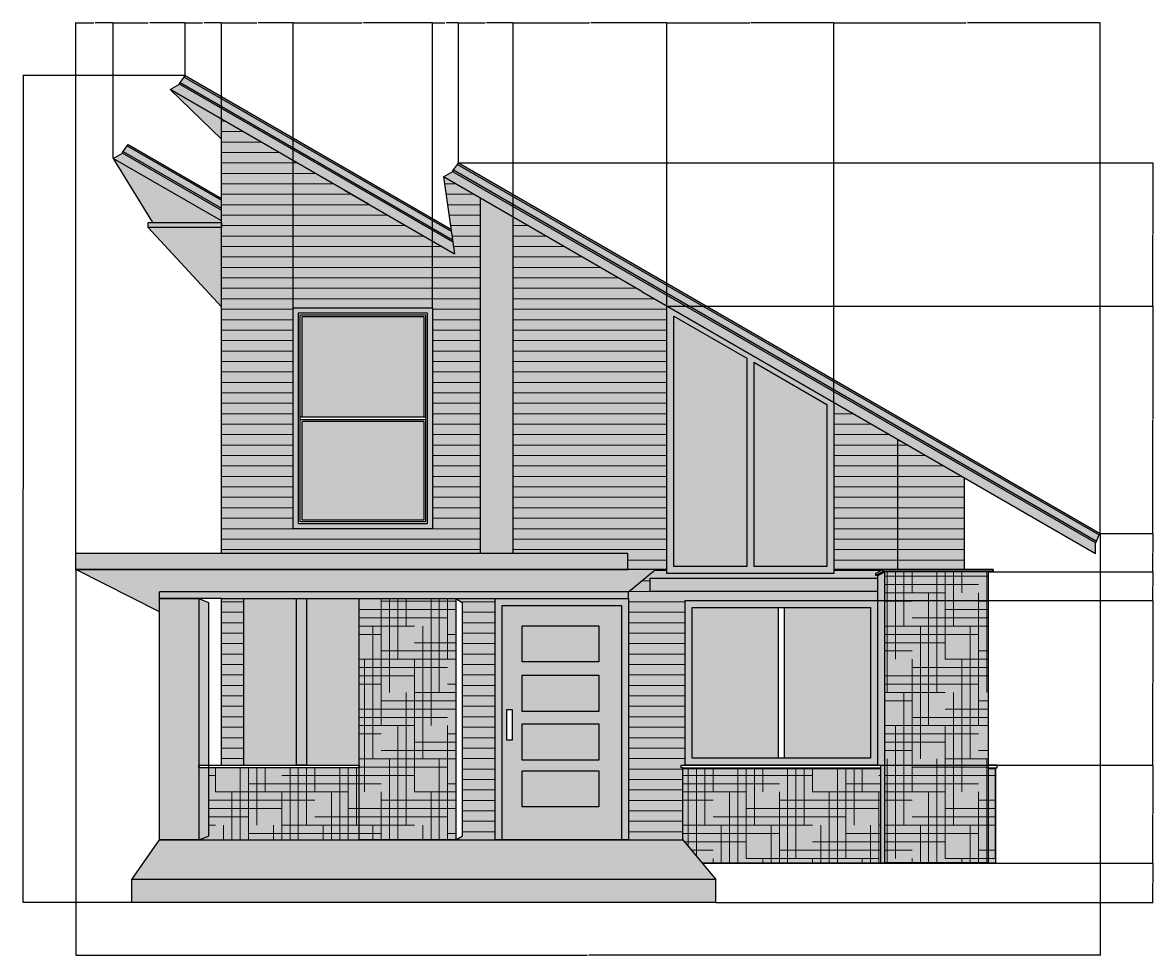
# Model space of a CAD drawing. Units: millimetres. Extents: x 171 to 1599, y 973 to 1509.
# Tile 1 of 7: x 171 to 821, y 973 to 1509. Entities that reach past the tile are written whole.
import ezdxf

# ---------------------------------------------------------------- set-up
doc = ezdxf.new("R2010")
doc.units = ezdxf.units.MM
for name, color, linetype, lineweight in [('A-ANNO-DIMS', 2, 'Continuous', 18), ('A-ELEV', 7, 'Continuous', 25), ('A-ELEV-FILL', 252, 'Continuous', 13), ('A-ELEV-PATT', 8, 'Continuous', 13)]:
    doc.layers.add(name, color=color, linetype=linetype, lineweight=lineweight)
doc.styles.get("Standard").update_dxf_attribs({"font": 'arial.ttf'})
doc.dimstyles.get("Standard").update_dxf_attribs({"dimtxt": 0.18, "dimasz": 0.18, "dimexe": 0.18, "dimexo": 0.0625, "dimgap": 0.09, "dimtad": 0, "dimtih": 1, "dimtoh": 1, "dimdec": 1, "dimzin": 0, "dimdsep": 46, "dimlunit": 3, "dimtxsty": 'Standard', "dimcen": 0.09, "dimadec": 0, "dimazin": 0, "dimtfac": 1, "dimtdec": 1, "dimtofl": 0, "dimtmove": 0, "dimatfit": 3, "dimfxl": 1, "dimtolj": 1, "dimtzin": 0, "dimarcsym": 0})
pattern_1 = [(0, (-1927.7, 0), (19.05, 4.7625), [76.2, -38.1]), (90, (-1927.7, 0), (-4.7625, -19.05), [76.2, -38.1])]

# ---------------------------------------------------------------- blocks, each defined once
blk = doc.blocks.new('*D19')
at = {"layer": 'A-ANNO-DIMS', "color": 0, "lineweight": -2, "transparency": 16777216}
for p, q in [((790.1, 1215.19), (790.1, 973)), ((202, 1194.43), (202, 973)), ((202.18, 973.18), (495.67, 973.18)), ((789.92, 973.18), (496.42, 973.18))]:
    blk.add_line(p, q, dxfattribs=at)
at = {"layer": 'A-ANNO-DIMS', "color": 0, "transparency": 16777216}
for points in [[(202.18, 973.21), (202.18, 973.15), (202, 973.18)], [(789.92, 973.21), (789.92, 973.15), (790.1, 973.18)]]:
    blk.add_solid(points, dxfattribs=at)
at = {"layer": 'Defpoints', "color": 0, "transparency": 16777216}
for p in [(790.1, 1215.25), (202, 1194.49), (790.1, 973.18)]:
    blk.add_point(p, dxfattribs=at)
at = {"layer": 'A-ANNO-DIMS', "color": 0, "transparency": 16777216, "insert": (496.05, 973.18), "char_height": 0.18, "attachment_point": 5}
blk.add_mtext('\\A1;588.1', dxfattribs=at)
blk = doc.blocks.new('*D20')
at = {"layer": 'A-ANNO-DIMS', "color": 0, "lineweight": -2, "transparency": 16777216}
for p, q in [((264.644382, 1478.130098), (171.566852, 1478.130098)), ((171.746852, 1477.950098), (171.746852, 1240.959874)), ((171.746852, 1003.60965), (171.746852, 1240.599874)), ((234.060756, 1003.42965), (171.566852, 1003.42965))]:
    blk.add_line(p, q, dxfattribs=at)
at = {"layer": 'A-ANNO-DIMS', "color": 0, "transparency": 16777216}
for points in [[(171.716852, 1477.950098), (171.776852, 1477.950098), (171.746852, 1478.130098)], [(171.716852, 1003.60965), (171.776852, 1003.60965), (171.746852, 1003.42965)]]:
    blk.add_solid(points, dxfattribs=at)
at = {"layer": 'Defpoints', "color": 0, "transparency": 16777216}
for p in [(171.746852, 1478.130098), (264.706882, 1478.130098), (234.123256, 1003.42965)]:
    blk.add_point(p, dxfattribs=at)
at = {"layer": 'A-ANNO-DIMS', "color": 0, "transparency": 16777216, "insert": (171.746852, 1240.779874), "char_height": 0.18, "attachment_point": 5}
blk.add_mtext('\\A1;474.7', dxfattribs=at)
blk = doc.blocks.new('*D21')
at = {"layer": 'A-ANNO-DIMS', "color": 0, "lineweight": -2, "transparency": 16777216}
for p, q in [((202, 1194.55), (202, 1508.56)), ((202.18, 1508.38), (212.26, 1508.38)), ((223.27, 1508.38), (213.19, 1508.38)), ((223.45, 1430.6), (223.45, 1508.56))]:
    blk.add_line(p, q, dxfattribs=at)
at = {"layer": 'A-ANNO-DIMS', "color": 0, "transparency": 16777216}
for points in [[(202.18, 1508.41), (202.18, 1508.35), (202, 1508.38)], [(223.27, 1508.41), (223.27, 1508.35), (223.45, 1508.38)]]:
    blk.add_solid(points, dxfattribs=at)
at = {"layer": 'Defpoints', "color": 0, "transparency": 16777216}
for p in [(223.45, 1508.38), (223.45, 1430.53), (202, 1194.49)]:
    blk.add_point(p, dxfattribs=at)
at = {"layer": 'A-ANNO-DIMS', "color": 0, "transparency": 16777216, "insert": (212.72, 1508.38), "char_height": 0.18, "attachment_point": 5}
blk.add_mtext('\\A1;21.455', dxfattribs=at)
blk = doc.blocks.new('*D22')
at = {"layer": 'A-ANNO-DIMS', "color": 0, "lineweight": -2, "transparency": 16777216}
for p, q in [((223.45, 1430.6), (223.45, 1508.56)), ((223.63, 1508.38), (243.61, 1508.38)), ((264.53, 1508.38), (244.55, 1508.38)), ((264.71, 1478.19), (264.71, 1508.56))]:
    blk.add_line(p, q, dxfattribs=at)
at = {"layer": 'A-ANNO-DIMS', "color": 0, "transparency": 16777216}
for points in [[(223.63, 1508.41), (223.63, 1508.35), (223.45, 1508.38)], [(264.53, 1508.41), (264.53, 1508.35), (264.71, 1508.38)]]:
    blk.add_solid(points, dxfattribs=at)
at = {"layer": 'Defpoints', "color": 0, "transparency": 16777216}
for p in [(264.71, 1508.38), (264.71, 1478.13), (223.45, 1430.53)]:
    blk.add_point(p, dxfattribs=at)
at = {"layer": 'A-ANNO-DIMS', "color": 0, "transparency": 16777216, "insert": (244.08, 1508.38), "char_height": 0.18, "attachment_point": 5}
blk.add_mtext('\\A1;41.255', dxfattribs=at)
blk = doc.blocks.new('*D23')
at = {"layer": 'A-ANNO-DIMS', "color": 0, "lineweight": -2, "transparency": 16777216}
for p, q in [((264.71, 1478.19), (264.71, 1508.56)), ((264.89, 1508.38), (274.67, 1508.38)), ((285.39, 1508.38), (275.61, 1508.38)), ((285.57, 1441.73), (285.57, 1508.56))]:
    blk.add_line(p, q, dxfattribs=at)
at = {"layer": 'A-ANNO-DIMS', "color": 0, "transparency": 16777216}
for points in [[(264.89, 1508.41), (264.89, 1508.35), (264.71, 1508.38)], [(285.39, 1508.41), (285.39, 1508.35), (285.57, 1508.38)]]:
    blk.add_solid(points, dxfattribs=at)
at = {"layer": 'Defpoints', "color": 0, "transparency": 16777216}
for p in [(285.57, 1508.38), (264.71, 1478.13), (285.57, 1441.66)]:
    blk.add_point(p, dxfattribs=at)
at = {"layer": 'A-ANNO-DIMS', "color": 0, "transparency": 16777216, "insert": (275.14, 1508.38), "char_height": 0.18, "attachment_point": 5}
blk.add_mtext('\\A1;20.865', dxfattribs=at)
blk = doc.blocks.new('*D24')
at = {"layer": 'A-ANNO-DIMS', "color": 0, "lineweight": -2, "transparency": 16777216}
for p, q in [((285.57, 1441.73), (285.57, 1508.56)), ((285.75, 1508.38), (305.85, 1508.38)), ((326.7, 1508.38), (306.61, 1508.38)), ((326.88, 1344.93), (326.88, 1508.56))]:
    blk.add_line(p, q, dxfattribs=at)
at = {"layer": 'A-ANNO-DIMS', "color": 0, "transparency": 16777216}
for points in [[(285.75, 1508.41), (285.75, 1508.35), (285.57, 1508.38)], [(326.7, 1508.41), (326.7, 1508.35), (326.88, 1508.38)]]:
    blk.add_solid(points, dxfattribs=at)
at = {"layer": 'Defpoints', "color": 0, "transparency": 16777216}
for p in [(326.88, 1508.38), (285.57, 1441.66), (326.88, 1344.87)]:
    blk.add_point(p, dxfattribs=at)
at = {"layer": 'A-ANNO-DIMS', "color": 0, "transparency": 16777216, "insert": (306.23, 1508.38), "char_height": 0.18, "attachment_point": 5}
blk.add_mtext('\\A1;41.31', dxfattribs=at)
blk = doc.blocks.new('*D25')
at = {"layer": 'A-ANNO-DIMS', "color": 0, "lineweight": -2, "transparency": 16777216}
for p, q in [((326.88, 1344.93), (326.88, 1508.56)), ((327.06, 1508.38), (366.45, 1508.38)), ((406.62, 1508.38), (367.23, 1508.38)), ((406.8, 1344.93), (406.8, 1508.56))]:
    blk.add_line(p, q, dxfattribs=at)
at = {"layer": 'A-ANNO-DIMS', "color": 0, "transparency": 16777216}
for points in [[(327.06, 1508.41), (327.06, 1508.35), (326.88, 1508.38)], [(406.62, 1508.41), (406.62, 1508.35), (406.8, 1508.38)]]:
    blk.add_solid(points, dxfattribs=at)
at = {"layer": 'Defpoints', "color": 0, "transparency": 16777216}
for p in [(406.8, 1508.38), (326.88, 1344.87), (406.8, 1344.87)]:
    blk.add_point(p, dxfattribs=at)
at = {"layer": 'A-ANNO-DIMS', "color": 0, "transparency": 16777216, "insert": (366.84, 1508.38), "char_height": 0.18, "attachment_point": 5}
blk.add_mtext('\\A1;79.92', dxfattribs=at)
blk = doc.blocks.new('*D26')
at = {"layer": 'A-ANNO-DIMS', "color": 0, "lineweight": -2, "transparency": 16777216}
for p, q in [((406.8, 1344.93), (406.8, 1508.56)), ((406.98, 1508.38), (413.85, 1508.38)), ((421.48, 1508.38), (414.62, 1508.38)), ((421.66, 1428.03), (421.66, 1508.56))]:
    blk.add_line(p, q, dxfattribs=at)
at = {"layer": 'A-ANNO-DIMS', "color": 0, "transparency": 16777216}
for points in [[(406.98, 1508.41), (406.98, 1508.35), (406.8, 1508.38)], [(421.48, 1508.41), (421.48, 1508.35), (421.66, 1508.38)]]:
    blk.add_solid(points, dxfattribs=at)
at = {"layer": 'Defpoints', "color": 0, "transparency": 16777216}
for p in [(421.66, 1508.38), (421.66, 1427.97), (406.8, 1344.87)]:
    blk.add_point(p, dxfattribs=at)
at = {"layer": 'A-ANNO-DIMS', "color": 0, "transparency": 16777216, "insert": (414.23, 1508.38), "char_height": 0.18, "attachment_point": 5}
blk.add_mtext('\\A1;14.86', dxfattribs=at)
blk = doc.blocks.new('*D27')
at = {"layer": 'A-ANNO-DIMS', "color": 0, "lineweight": -2, "transparency": 16777216}
for p, q in [((421.66, 1428.03), (421.66, 1508.56)), ((421.84, 1508.38), (436.95, 1508.38)), ((452.99, 1508.38), (437.88, 1508.38)), ((453.17, 1396.85), (453.17, 1508.56))]:
    blk.add_line(p, q, dxfattribs=at)
at = {"layer": 'A-ANNO-DIMS', "color": 0, "transparency": 16777216}
for points in [[(421.84, 1508.41), (421.84, 1508.35), (421.66, 1508.38)], [(452.99, 1508.41), (452.99, 1508.35), (453.17, 1508.38)]]:
    blk.add_solid(points, dxfattribs=at)
at = {"layer": 'Defpoints', "color": 0, "transparency": 16777216}
for p in [(453.17, 1508.38), (421.66, 1427.97), (453.17, 1396.79)]:
    blk.add_point(p, dxfattribs=at)
at = {"layer": 'A-ANNO-DIMS', "color": 0, "transparency": 16777216, "insert": (437.41, 1508.38), "char_height": 0.18, "attachment_point": 5}
blk.add_mtext('\\A1;31.505', dxfattribs=at)
blk = doc.blocks.new('*D28')
at = {"layer": 'A-ANNO-DIMS', "color": 0, "lineweight": -2, "transparency": 16777216}
for p, q in [((453.17, 1396.85), (453.17, 1508.56)), ((453.35, 1508.38), (496.88, 1508.38)), ((541.21, 1508.38), (497.67, 1508.38)), ((541.39, 1345.92), (541.39, 1508.56))]:
    blk.add_line(p, q, dxfattribs=at)
at = {"layer": 'A-ANNO-DIMS', "color": 0, "transparency": 16777216}
for points in [[(453.35, 1508.41), (453.35, 1508.35), (453.17, 1508.38)], [(541.21, 1508.41), (541.21, 1508.35), (541.39, 1508.38)]]:
    blk.add_solid(points, dxfattribs=at)
at = {"layer": 'Defpoints', "color": 0, "transparency": 16777216}
for p in [(541.39, 1508.38), (453.17, 1396.79), (541.39, 1345.85)]:
    blk.add_point(p, dxfattribs=at)
at = {"layer": 'A-ANNO-DIMS', "color": 0, "transparency": 16777216, "insert": (497.28, 1508.38), "char_height": 0.18, "attachment_point": 5}
blk.add_mtext('\\A1;88.22', dxfattribs=at)
blk = doc.blocks.new('*D29')
at = {"layer": 'A-ANNO-DIMS', "color": 0, "lineweight": -2, "transparency": 16777216}
for p, q in [((541.39, 1345.92), (541.39, 1508.56)), ((541.57, 1508.38), (589.01, 1508.38)), ((637.11, 1508.38), (589.66, 1508.38)), ((637.29, 1290.55), (637.29, 1508.56))]:
    blk.add_line(p, q, dxfattribs=at)
at = {"layer": 'A-ANNO-DIMS', "color": 0, "transparency": 16777216}
for points in [[(541.57, 1508.41), (541.57, 1508.35), (541.39, 1508.38)], [(637.11, 1508.41), (637.11, 1508.35), (637.29, 1508.38)]]:
    blk.add_solid(points, dxfattribs=at)
at = {"layer": 'Defpoints', "color": 0, "transparency": 16777216}
for p in [(637.29, 1508.38), (541.39, 1345.85), (637.29, 1290.48)]:
    blk.add_point(p, dxfattribs=at)
at = {"layer": 'A-ANNO-DIMS', "color": 0, "transparency": 16777216, "insert": (589.34, 1508.38), "char_height": 0.18, "attachment_point": 5}
blk.add_mtext('\\A1;95.9', dxfattribs=at)
blk = doc.blocks.new('*D30')
at = {"layer": 'A-ANNO-DIMS', "color": 0, "lineweight": -2, "transparency": 16777216}
for p, q in [((637.29, 1290.55), (637.29, 1508.56)), ((637.47, 1508.38), (713.31, 1508.38)), ((789.92, 1508.38), (714.08, 1508.38)), ((790.1, 1215.31), (790.1, 1508.56))]:
    blk.add_line(p, q, dxfattribs=at)
at = {"layer": 'A-ANNO-DIMS', "color": 0, "transparency": 16777216}
for points in [[(637.47, 1508.41), (637.47, 1508.35), (637.29, 1508.38)], [(789.92, 1508.41), (789.92, 1508.35), (790.1, 1508.38)]]:
    blk.add_solid(points, dxfattribs=at)
at = {"layer": 'Defpoints', "color": 0, "transparency": 16777216}
for p in [(790.1, 1508.38), (637.29, 1290.48), (790.1, 1215.25)]:
    blk.add_point(p, dxfattribs=at)
at = {"layer": 'A-ANNO-DIMS', "color": 0, "transparency": 16777216, "insert": (713.69, 1508.38), "char_height": 0.18, "attachment_point": 5}
blk.add_mtext('\\A1;152.8', dxfattribs=at)
blk = doc.blocks.new('*D31')
at = {"layer": 'A-ANNO-DIMS', "color": 0, "lineweight": -2, "transparency": 16777216}
for p, q in [((730.2, 1026.04), (820.53, 1026.04)), ((820.35, 1025.86), (820.35, 1014.92)), ((820.35, 1003.61), (820.35, 1014.55)), ((569.52, 1003.43), (820.53, 1003.43))]:
    blk.add_line(p, q, dxfattribs=at)
at = {"layer": 'A-ANNO-DIMS', "color": 0, "transparency": 16777216}
for points in [[(820.32, 1025.86), (820.38, 1025.86), (820.35, 1026.04)], [(820.32, 1003.61), (820.38, 1003.61), (820.35, 1003.43)]]:
    blk.add_solid(points, dxfattribs=at)
at = {"layer": 'Defpoints', "color": 0, "transparency": 16777216}
for p in [(730.13, 1026.04), (820.35, 1026.04), (569.45, 1003.43)]:
    blk.add_point(p, dxfattribs=at)
at = {"layer": 'A-ANNO-DIMS', "color": 0, "transparency": 16777216, "insert": (820.35, 1014.73), "char_height": 0.18, "attachment_point": 5}
blk.add_mtext('\\A1;22.61', dxfattribs=at)
blk = doc.blocks.new('*D32')
at = {"layer": 'A-ANNO-DIMS', "color": 0, "lineweight": -2, "transparency": 16777216}
for p, q in [((662.41, 1082.23), (820.53, 1082.23)), ((820.35, 1082.05), (820.35, 1054.32)), ((820.35, 1026.22), (820.35, 1053.95)), ((730.2, 1026.04), (820.53, 1026.04))]:
    blk.add_line(p, q, dxfattribs=at)
at = {"layer": 'A-ANNO-DIMS', "color": 0, "transparency": 16777216}
for points in [[(820.32, 1082.05), (820.38, 1082.05), (820.35, 1082.23)], [(820.32, 1026.22), (820.38, 1026.22), (820.35, 1026.04)]]:
    blk.add_solid(points, dxfattribs=at)
at = {"layer": 'Defpoints', "color": 0, "transparency": 16777216}
for p in [(662.34, 1082.23), (820.35, 1082.23), (730.13, 1026.04)]:
    blk.add_point(p, dxfattribs=at)
at = {"layer": 'A-ANNO-DIMS', "color": 0, "transparency": 16777216, "insert": (820.35, 1054.14), "char_height": 0.18, "attachment_point": 5}
blk.add_mtext('\\A1;56.19', dxfattribs=at)
blk = doc.blocks.new('*D33')
at = {"layer": 'A-ANNO-DIMS', "color": 0, "lineweight": -2, "transparency": 16777216}
for p, q in [((662.41, 1176.74), (820.53, 1176.74)), ((820.35, 1176.56), (820.35, 1129.67)), ((820.35, 1082.41), (820.35, 1129.31)), ((662.41, 1082.23), (820.53, 1082.23))]:
    blk.add_line(p, q, dxfattribs=at)
at = {"layer": 'A-ANNO-DIMS', "color": 0, "transparency": 16777216}
for points in [[(820.32, 1176.56), (820.38, 1176.56), (820.35, 1176.74)], [(820.32, 1082.41), (820.38, 1082.41), (820.35, 1082.23)]]:
    blk.add_solid(points, dxfattribs=at)
at = {"layer": 'Defpoints', "color": 0, "transparency": 16777216}
for p in [(662.34, 1176.74), (820.35, 1176.74), (662.34, 1082.23)]:
    blk.add_point(p, dxfattribs=at)
at = {"layer": 'A-ANNO-DIMS', "color": 0, "transparency": 16777216, "insert": (820.35, 1129.49), "char_height": 0.18, "attachment_point": 5}
blk.add_mtext('\\A1;94.51', dxfattribs=at)
blk = doc.blocks.new('*D34')
at = {"layer": 'A-ANNO-DIMS', "color": 0, "lineweight": -2, "transparency": 16777216}
for p, q in [((725.9, 1193.22), (820.53, 1193.22)), ((820.35, 1193.04), (820.35, 1185.16)), ((820.35, 1176.92), (820.35, 1184.8)), ((662.41, 1176.74), (820.53, 1176.74))]:
    blk.add_line(p, q, dxfattribs=at)
at = {"layer": 'A-ANNO-DIMS', "color": 0, "transparency": 16777216}
for points in [[(820.32, 1193.04), (820.38, 1193.04), (820.35, 1193.22)], [(820.32, 1176.92), (820.38, 1176.92), (820.35, 1176.74)]]:
    blk.add_solid(points, dxfattribs=at)
at = {"layer": 'Defpoints', "color": 0, "transparency": 16777216}
for p in [(725.84, 1193.22), (820.35, 1193.22), (662.34, 1176.74)]:
    blk.add_point(p, dxfattribs=at)
at = {"layer": 'A-ANNO-DIMS', "color": 0, "transparency": 16777216, "insert": (820.35, 1184.98), "char_height": 0.18, "attachment_point": 5}
blk.add_mtext('\\A1;16.478', dxfattribs=at)
blk = doc.blocks.new('*D35')
at = {"layer": 'A-ANNO-DIMS', "color": 0, "lineweight": -2, "transparency": 16777216}
for p, q in [((790.16, 1215.25), (820.53, 1215.25)), ((820.35, 1215.07), (820.35, 1204.42)), ((820.35, 1193.4), (820.35, 1204.05)), ((725.9, 1193.22), (820.53, 1193.22))]:
    blk.add_line(p, q, dxfattribs=at)
at = {"layer": 'A-ANNO-DIMS', "color": 0, "transparency": 16777216}
for points in [[(820.32, 1215.07), (820.38, 1215.07), (820.35, 1215.25)], [(820.32, 1193.4), (820.38, 1193.4), (820.35, 1193.22)]]:
    blk.add_solid(points, dxfattribs=at)
at = {"layer": 'Defpoints', "color": 0, "transparency": 16777216}
for p in [(790.1, 1215.25), (820.35, 1215.25), (725.84, 1193.22)]:
    blk.add_point(p, dxfattribs=at)
at = {"layer": 'A-ANNO-DIMS', "color": 0, "transparency": 16777216, "insert": (820.35, 1204.24), "char_height": 0.18, "attachment_point": 5}
blk.add_mtext('\\A1;22.03', dxfattribs=at)
blk = doc.blocks.new('*D36')
at = {"layer": 'A-ANNO-DIMS', "color": 0, "lineweight": -2, "transparency": 16777216}
for p, q in [((541.45, 1345.85), (820.53, 1345.85)), ((820.35, 1345.67), (820.35, 1280.73)), ((820.35, 1215.43), (820.35, 1280.37)), ((790.16, 1215.25), (820.53, 1215.25))]:
    blk.add_line(p, q, dxfattribs=at)
at = {"layer": 'A-ANNO-DIMS', "color": 0, "transparency": 16777216}
for points in [[(820.32, 1345.67), (820.38, 1345.67), (820.35, 1345.85)], [(820.32, 1215.43), (820.38, 1215.43), (820.35, 1215.25)]]:
    blk.add_solid(points, dxfattribs=at)
at = {"layer": 'Defpoints', "color": 0, "transparency": 16777216}
for p in [(541.39, 1345.85), (820.35, 1345.85), (790.1, 1215.25)]:
    blk.add_point(p, dxfattribs=at)
at = {"layer": 'A-ANNO-DIMS', "color": 0, "transparency": 16777216, "insert": (820.35, 1280.55), "char_height": 0.18, "attachment_point": 5}
blk.add_mtext('\\A1;130.6', dxfattribs=at)
blk = doc.blocks.new('*D37')
at = {"layer": 'A-ANNO-DIMS', "color": 0, "lineweight": -2, "transparency": 16777216}
for p, q in [((421.72, 1427.97), (820.53, 1427.97)), ((820.35, 1427.79), (820.35, 1387.09)), ((820.35, 1346.03), (820.35, 1386.73)), ((541.45, 1345.85), (820.53, 1345.85))]:
    blk.add_line(p, q, dxfattribs=at)
at = {"layer": 'A-ANNO-DIMS', "color": 0, "transparency": 16777216}
for points in [[(820.32, 1427.79), (820.38, 1427.79), (820.35, 1427.97)], [(820.32, 1346.03), (820.38, 1346.03), (820.35, 1345.85)]]:
    blk.add_solid(points, dxfattribs=at)
at = {"layer": 'Defpoints', "color": 0, "transparency": 16777216}
for p in [(421.66, 1427.97), (820.35, 1427.97), (541.39, 1345.85)]:
    blk.add_point(p, dxfattribs=at)
at = {"layer": 'A-ANNO-DIMS', "color": 0, "transparency": 16777216, "insert": (820.35, 1386.91), "char_height": 0.18, "attachment_point": 5}
blk.add_mtext('\\A1;82.12', dxfattribs=at)

msp = doc.modelspace()

# ---------------------------------------------------------------- hatches: boundary and pattern name
at = {"layer": 'A-ELEV-FILL'}
h = msp.add_hatch(color=256, dxfattribs=at)
h.dxf.hatch_style = 1
h.paths.add_polyline_path([(231.7811, 1438.5737), (231.309, 1437.7559), (285.3227, 1406.5711), (285.3227, 1407.6614)])
h.paths.add_polyline_path([(231.309, 1437.7559), (228.8893, 1434.5494), (285.3227, 1401.9675), (285.3227, 1406.5711)])
h.paths.add_polyline_path([(228.58, 1433.6376), (223.2033, 1430.5334), (285.3227, 1394.6687), (285.3227, 1400.8772)])
h.paths.add_polyline_path([(228.8893, 1434.5494), (228.363, 1433.7629), (285.3227, 1400.8772), (285.3227, 1401.9675)])
h.paths.add_polyline_path([(285.3227, 1393.7984), (243.3138, 1393.7984), (243.3138, 1390.8634), (285.3227, 1390.8634)])
h.paths.add_polyline_path([(261.2571, 1473.194), (255.8803, 1470.0898), (369.7228, 1404.3628), (419.1117, 1375.8481), (418.1483, 1382.6128)])
h.paths.add_polyline_path([(261.5664, 1474.1058), (261.0401, 1473.3193), (418.1483, 1382.6128), (417.9791, 1383.8008)])
h.paths.add_polyline_path([(263.986, 1477.3124), (261.5664, 1474.1058), (417.9791, 1383.8008), (417.2648, 1388.8168)])
h.paths.add_polyline_path([(264.4581, 1478.1301), (263.986, 1477.3124), (417.2648, 1388.8168), (417.0956, 1390.0048)])
h.paths.add_polyline_path([(418.2107, 1423.034), (412.834, 1419.9297), (526.6765, 1354.2027), (787.1762, 1203.8031), (787.1762, 1210.0116)])
h.paths.add_polyline_path([(420.9397, 1427.1523), (418.52, 1423.9457), (787.8112, 1210.7354), (789.3783, 1214.4341)])
h.paths.add_polyline_path([(421.4118, 1427.97), (420.9397, 1427.1523), (789.3783, 1214.4341), (789.8504, 1215.2519)])
h.paths.add_polyline_path([(418.52, 1423.9457), (417.9937, 1423.1592), (787.3932, 1209.8864), (787.8112, 1210.7354)])
h = msp.add_hatch(color=256, dxfattribs=at)
h.dxf.hatch_style = 1
h.paths.add_polyline_path([(285.3227, 1390.8634), (243.3138, 1390.8634), (285.3227, 1345.3593)])
h.paths.add_polyline_path([(223.2033, 1430.5334), (245.7908, 1393.7984), (285.3227, 1393.7984), (285.3227, 1394.6687)])
h.paths.add_polyline_path([(255.8803, 1470.0898), (285.3227, 1441.6631), (285.3227, 1453.0912)])
h.paths.add_polyline_path([(434.1666, 1407.6133), (412.834, 1419.9297), (419.1117, 1375.8481), (434.1666, 1367.1562)])
h.paths.add_polyline_path([(452.9171, 1396.7877), (434.1666, 1407.6133), (434.1666, 1203.7941), (452.9171, 1203.7941)])
h.paths.add_polyline_path([(402.5524, 1282.2145), (330.6353, 1282.2145), (330.6353, 1280.5242), (402.5524, 1280.5242)], flags=0)
h.paths.add_polyline_path([(402.5524, 1280.5242), (330.6353, 1280.5242), (330.6353, 1221.867), (402.5524, 1221.867)], flags=0)
h.paths.add_polyline_path([(401.5524, 1279.5242), (401.5524, 1222.867), (331.6353, 1222.867), (331.6353, 1279.5242)], flags=0)
h.paths.add_polyline_path([(406.5524, 1344.8717), (326.6353, 1344.8717), (326.6353, 1217.867), (406.5524, 1217.867)])
h.paths.add_polyline_path([(403.5524, 1341.8717), (403.5524, 1220.867), (329.6353, 1220.867), (329.6353, 1341.8717)], flags=0)
h.paths.add_polyline_path([(402.5524, 1340.8717), (402.5524, 1221.867), (330.6353, 1221.867), (330.6353, 1340.8717)], flags=0)
h.paths.add_polyline_path([(401.5524, 1339.8717), (401.5524, 1282.2145), (402.5524, 1282.2145), (402.5524, 1280.5242), (330.6353, 1280.5242), (330.6353, 1282.2145), (331.6353, 1282.2145), (331.6353, 1339.8717)], flags=0)
h.paths.add_polyline_path([(403.5524, 1341.8717), (329.6353, 1341.8717), (329.6353, 1220.867), (403.5524, 1220.867)], flags=16)
h.paths.add_polyline_path([(331.6353, 1339.8717), (401.5524, 1339.8717), (401.5524, 1282.2145), (402.5524, 1282.2145), (402.5524, 1340.8717), (330.6353, 1340.8717), (330.6353, 1282.2145), (331.6353, 1282.2145)], flags=0)
h.paths.add_polyline_path([(637.0394, 1290.4846), (541.1379, 1345.8534), (541.1379, 1192.267), (637.0394, 1192.267)])
h.paths.add_polyline_path([(587.0887, 1196.267), (545.1379, 1196.267), (545.1379, 1340.0799), (587.0887, 1315.8596)], flags=16)
h.paths.add_polyline_path([(591.0887, 1313.5502), (633.0394, 1289.3299), (633.0394, 1196.267), (591.0887, 1196.267)], flags=16)
h.paths.add_polyline_path([(662.0939, 1189.6048), (531.4556, 1189.6048), (531.4556, 1181.9686), (662.0939, 1181.9686)])
h.paths.add_polyline_path([(662.0939, 1176.7441), (551.7144, 1176.7441), (551.7144, 1082.2327), (662.0939, 1082.2327)])
h.paths.add_polyline_path([(658.0939, 1172.7441), (658.0939, 1086.2327), (555.7144, 1086.2327), (555.7144, 1172.7441)], flags=16)
h.paths.add_polyline_path([(608.5162, 1172.7441), (605.2921, 1172.7441), (605.2921, 1086.2327), (608.5162, 1086.2327)], flags=0)
h.paths.add_polyline_path([(519.0541, 1177.8722), (442.5372, 1177.8722), (442.5372, 1039.2493), (446.5372, 1039.2493), (446.5372, 1173.8722), (515.0541, 1173.8722), (515.0541, 1039.2493), (519.0541, 1039.2493)])
h.paths.add_polyline_path([(272.4403, 1177.8722), (249.8847, 1177.8722), (249.8847, 1039.2493), (272.4403, 1039.2493)])
h.paths.add_polyline_path([(277.9553, 1175.6512), (272.4403, 1177.8722), (272.4403, 1082.2327), (277.9553, 1082.2327)])
h.paths.add_polyline_path([(518.6551, 1203.7941), (201.7481, 1203.7941), (201.7481, 1194.488), (518.6551, 1194.488)])
h.paths.add_polyline_path([(334.2275, 1177.8722), (328.3807, 1177.8722), (328.3807, 1082.2327), (334.2275, 1082.2327)])
h.paths.add_polyline_path([(519.0541, 1181.6916), (285.3227, 1181.6916), (249.8847, 1181.6916), (249.8847, 1177.8722), (285.3227, 1177.8722), (519.0541, 1177.8722)])
h = msp.add_hatch(color=256, dxfattribs=at)
h.dxf.hatch_style = 1
h.paths.add_polyline_path([(355.9834, 1412.2952), (285.3227, 1453.0912), (285.3227, 1203.7941), (434.1666, 1203.7941), (434.1666, 1367.1562)])
h.paths.add_polyline_path([(326.6353, 1344.8717), (406.5524, 1344.8717), (406.5524, 1217.867), (326.6353, 1217.867)], flags=16)
h.paths.add_polyline_path([(329.6353, 1341.8717), (403.5524, 1341.8717), (403.5524, 1220.867), (329.6353, 1220.867)], flags=0)
h.paths.add_polyline_path([(330.6353, 1340.8717), (402.5524, 1340.8717), (402.5524, 1221.867), (330.6353, 1221.867)], flags=0)
h.paths.add_polyline_path([(331.6353, 1339.8717), (401.5524, 1339.8717), (401.5524, 1282.2145), (402.5524, 1282.2145), (402.5524, 1280.5242), (330.6353, 1280.5242), (330.6353, 1282.2145), (331.6353, 1282.2145)], flags=0)
h.paths.add_polyline_path([(331.6353, 1279.5242), (401.5524, 1279.5242), (401.5524, 1222.867), (331.6353, 1222.867)], flags=0)
h.paths.add_polyline_path([(541.1379, 1345.8534), (526.6765, 1354.2027), (452.9171, 1396.7877), (452.9171, 1203.7941), (518.6551, 1203.7941), (518.6551, 1194.488), (541.1379, 1194.488)])
h.paths.add_polyline_path([(298.0899, 1177.8722), (285.3227, 1177.8722), (285.3227, 1082.2327), (298.0899, 1082.2327)])
h.paths.add_polyline_path([(711.831, 1247.3037), (673.6749, 1269.3331), (673.6749, 1194.488), (711.831, 1194.488)])
h.paths.add_polyline_path([(673.6749, 1269.3331), (637.0394, 1290.4846), (637.0394, 1194.488), (665.0967, 1194.488), (673.6749, 1194.488)])
h.paths.add_polyline_path([(551.7144, 1176.7441), (662.0939, 1176.7441), (662.0939, 1181.9686), (531.4556, 1181.9686), (531.4556, 1189.6048), (662.0939, 1189.6048), (662.0939, 1191.2497), (660.9467, 1191.2497), (660.9467, 1192.267), (665.0967, 1194.488), (637.0394, 1194.488), (637.0394, 1192.267), (541.1379, 1192.267), (541.1379, 1194.488), (534.6535, 1194.488), (519.0541, 1181.6916), (519.0541, 1177.8722), (519.0541, 1039.2493), (550.258, 1039.2493), (550.258, 1080.6718), (549.2915, 1080.6718), (549.2915, 1082.2327), (551.7144, 1082.2327)])
h.paths.add_polyline_path([(442.5372, 1177.8722), (419.9268, 1177.8722), (423.6566, 1175.6512), (423.6566, 1041.4702), (419.9268, 1039.2493), (442.5372, 1039.2493)])
h = msp.add_hatch(color=256, dxfattribs=at)
h.dxf.hatch_style = 1
h.paths.add_polyline_path([(401.5524, 1339.8717), (331.6353, 1339.8717), (331.6353, 1282.2145), (401.5524, 1282.2145)])
h.paths.add_polyline_path([(401.5524, 1279.5242), (331.6353, 1279.5242), (331.6353, 1222.867), (401.5524, 1222.867)])
h.paths.add_polyline_path([(633.0394, 1289.3299), (591.0887, 1313.5502), (591.0887, 1196.267), (633.0394, 1196.267)])
h.paths.add_polyline_path([(587.0887, 1315.8596), (545.1379, 1340.0799), (545.1379, 1196.267), (587.0887, 1196.267)])
h.paths.add_polyline_path([(658.0939, 1172.7441), (608.5162, 1172.7441), (608.5162, 1086.2327), (658.0939, 1086.2327)])
h.paths.add_polyline_path([(605.2921, 1172.7441), (555.7144, 1172.7441), (555.7144, 1086.2327), (605.2921, 1086.2327)])
h.paths.add_polyline_path([(328.3807, 1177.8722), (298.0899, 1177.8722), (298.0899, 1082.2327), (328.3807, 1082.2327)])
h.paths.add_polyline_path([(364.5178, 1177.8722), (334.2275, 1177.8722), (334.2275, 1082.2327), (364.5178, 1082.2327)])
h.paths.add_polyline_path([(502.0594, 1162.2854), (458.1261, 1162.2854), (458.1261, 1141.4523), (502.0594, 1141.4523)])
h.paths.add_polyline_path([(502.0594, 1133.885), (458.1261, 1133.885), (458.1261, 1113.0519), (502.0594, 1113.0519)])
h.paths.add_polyline_path([(502.0594, 1105.9503), (458.1261, 1105.9503), (458.1261, 1085.1172), (502.0594, 1085.1172)])
h.paths.add_polyline_path([(502.0594, 1079.0383), (458.1261, 1079.0383), (458.1261, 1058.2052), (502.0594, 1058.2052)])
h = msp.add_hatch(color=256, dxfattribs=at)
h.dxf.hatch_style = 1
h.paths.add_polyline_path([(534.6535, 1194.488), (201.7481, 1194.488), (249.8847, 1170.1702), (249.8847, 1177.8722), (249.8847, 1181.6916), (285.3227, 1181.6916), (519.0541, 1181.6916)])
h = msp.add_hatch(color=256, dxfattribs=at)
h.dxf.hatch_style = 1
h.paths.add_polyline_path([(419.9268, 1177.8722), (364.5178, 1177.8722), (364.5178, 1039.2493), (419.9268, 1039.2493)])
h.paths.add_polyline_path([(364.5178, 1080.6718), (277.9553, 1080.6718), (277.9553, 1041.4702), (272.4403, 1039.2493), (364.5178, 1039.2493)])
h.paths.add_polyline_path([(277.9553, 1080.6718), (272.4403, 1080.6718), (272.4403, 1039.2493), (277.9553, 1041.4702)], flags=17)
h.paths.add_polyline_path([(550.258, 1039.2493), (249.8847, 1039.2493), (233.8745, 1016.6402), (569.2044, 1016.6402)])
h.paths.add_polyline_path([(569.2044, 1016.6402), (233.8745, 1016.6402), (233.8745, 1003.4297), (569.2044, 1003.4297)])
h.paths.add_polyline_path([(725.5866, 1193.222), (666.2439, 1193.222), (666.2439, 1026.0766), (725.5866, 1026.0766)])
h.paths.add_polyline_path([(664.015, 1080.3893), (550.258, 1080.3893), (550.258, 1039.2493), (561.3284, 1026.0387), (664.015, 1026.0387)])
h.paths.add_polyline_path([(729.8847, 1080.3893), (725.5866, 1080.3893), (725.5866, 1026.0387), (729.8847, 1026.0387)])
h.paths.add_polyline_path([(666.2439, 1193.222), (662.0939, 1191.0011), (662.0939, 1082.2327), (664.015, 1082.2327), (664.015, 1026.0387), (666.2439, 1026.0387)])
h = msp.add_hatch(color=256, dxfattribs=at)
h.dxf.hatch_style = 1
h.paths.add_polyline_path([(515.0541, 1173.8722), (446.5372, 1173.8722), (446.5372, 1039.2493), (515.0541, 1039.2493)])
h.paths.add_polyline_path([(502.0594, 1162.2854), (502.0594, 1141.4523), (458.1261, 1141.4523), (458.1261, 1162.2854)], flags=16)
h.paths.add_polyline_path([(502.0594, 1133.885), (502.0594, 1113.0519), (458.1261, 1113.0519), (458.1261, 1133.885)], flags=16)
h.paths.add_polyline_path([(452.2763, 1114.2546), (452.2763, 1096.495), (449.2169, 1096.495), (449.2169, 1114.2546)], flags=16)
h.paths.add_polyline_path([(502.0594, 1105.9503), (502.0594, 1085.1172), (458.1261, 1085.1172), (458.1261, 1105.9503)], flags=16)
h.paths.add_polyline_path([(502.0594, 1079.0383), (502.0594, 1058.2052), (458.1261, 1058.2052), (458.1261, 1079.0383)], flags=16)
at = {"layer": 'A-ELEV-PATT'}
h = msp.add_hatch(dxfattribs=at)
h.set_pattern_fill('_USER', color=256, scale=6, pattern_type=0)
h.set_pattern_definition([(0, (-1927.7, 0), (0, 6), [])])
h.paths.add_polyline_path([(434.4153, 1407.6133), (413.0827, 1419.9297), (419.3604, 1375.8481), (356.2322, 1412.2952), (285.5715, 1453.0912), (285.5715, 1203.7941), (434.4153, 1203.7941)])
h.paths.add_polyline_path([(326.8841, 1344.8717), (406.8011, 1344.8717), (406.8011, 1217.867), (326.8841, 1217.867)], flags=16)
h.paths.add_polyline_path([(329.8841, 1341.8717), (403.8011, 1341.8717), (403.8011, 1220.867), (329.8841, 1220.867)], flags=0)
h.paths.add_polyline_path([(330.8841, 1340.8717), (402.8011, 1340.8717), (402.8011, 1221.867), (330.8841, 1221.867)], flags=0)
h.paths.add_polyline_path([(331.8841, 1339.8717), (401.8011, 1339.8717), (401.8011, 1282.2145), (402.8011, 1282.2145), (402.8011, 1280.5242), (330.8841, 1280.5242), (330.8841, 1282.2145), (331.8841, 1282.2145)], flags=0)
h.paths.add_polyline_path([(331.8841, 1279.5242), (401.8011, 1279.5242), (401.8011, 1222.867), (331.8841, 1222.867)], flags=0)
h.paths.add_polyline_path([(541.3866, 1345.8534), (526.9252, 1354.2027), (453.1658, 1396.7877), (453.1658, 1203.7941), (518.9039, 1203.7941), (518.9039, 1194.488), (541.3866, 1194.488)])
h.paths.add_polyline_path([(673.9237, 1269.3331), (637.2881, 1290.4846), (637.2881, 1194.488), (665.3454, 1194.488), (673.9237, 1194.488)])
h.paths.add_polyline_path([(712.0797, 1247.3037), (673.9237, 1269.3331), (673.9237, 1194.488), (712.0797, 1194.488)])
h.paths.add_polyline_path([(298.3386, 1177.8722), (285.5715, 1177.8722), (285.5715, 1082.2327), (298.3386, 1082.2327)])
h.paths.add_polyline_path([(442.7859, 1177.8722), (420.1756, 1177.8722), (423.9053, 1175.6512), (423.9053, 1041.4702), (420.1756, 1039.2493), (442.7859, 1039.2493)])
h.paths.add_polyline_path([(551.9631, 1176.7441), (662.3427, 1176.7441), (662.3427, 1181.9686), (531.7043, 1181.9686), (531.7043, 1189.6048), (662.3427, 1189.6048), (662.3427, 1191.2497), (661.1955, 1191.2497), (661.1955, 1192.267), (665.3454, 1194.488), (637.2881, 1194.488), (637.2881, 1192.267), (541.3866, 1192.267), (541.3866, 1194.488), (534.9023, 1194.488), (519.3028, 1181.6916), (519.3028, 1177.8722), (519.3028, 1039.2493), (550.5068, 1039.2493), (550.5068, 1080.6718), (549.5402, 1080.6718), (549.5402, 1082.2327), (551.9631, 1082.2327)])
h = msp.add_hatch(dxfattribs=at)
h.set_pattern_fill('HOUND', color=256, scale=3)
h.set_pattern_definition(pattern_1)
h.paths.add_polyline_path([(364.7665, 1080.6718), (278.204, 1080.6718), (278.204, 1041.4702), (272.6891, 1039.2493), (364.7665, 1039.2493)])
h.paths.add_polyline_path([(725.8354, 1193.222), (666.4926, 1193.222), (666.4926, 1026.0766), (725.8354, 1026.0766)])
h.paths.add_polyline_path([(664.2637, 1080.3893), (550.5068, 1080.3893), (550.5068, 1039.2493), (561.5772, 1026.0387), (664.2637, 1026.0387)])
h.paths.add_polyline_path([(730.1334, 1080.3893), (725.8354, 1080.3893), (725.8354, 1026.0387), (730.1334, 1026.0387)])
h = msp.add_hatch(dxfattribs=at)
h.set_pattern_fill('HOUND', color=256, scale=3)
h.set_pattern_definition(pattern_1)
h.paths.add_polyline_path([(420.1756, 1177.8722), (364.7665, 1177.8722), (364.7665, 1039.2493), (420.1756, 1039.2493)])

# ---------------------------------------------------------------- linework, layer by layer
at = {"layer": 'A-ELEV'}
for p, q in [((261.2888, 1473.3193), (261.8151, 1474.1058)), ((261.8151, 1474.1058), (264.2348, 1477.3124)), ((261.8151, 1474.1058), (418.2279, 1383.8008)), ((264.2348, 1477.3124), (264.7069, 1478.1301)), ((264.2348, 1477.3124), (417.5135, 1388.8168)), ((264.7069, 1478.1301), (417.3443, 1390.0048)), ((256.1291, 1470.0898), (261.5058, 1473.194)), ((369.9716, 1404.3628), (256.1291, 1470.0898)), ((256.1291, 1470.0898), (285.5715, 1441.6631)), ((261.2888, 1473.3193), (418.397, 1382.6128)), ((261.5058, 1473.194), (261.2888, 1473.3193)), ((285.5715, 1203.7941), (285.5715, 1453.0912)), ((229.138, 1434.5494), (231.5577, 1437.7559)), ((231.5577, 1437.7559), (232.0298, 1438.5737)), ((231.5577, 1437.7559), (285.5715, 1406.5711)), ((232.0298, 1438.5737), (285.5715, 1407.6614)), ((223.452, 1430.5334), (228.8287, 1433.6376)), ((285.5715, 1394.6687), (223.452, 1430.5334)), ((223.452, 1430.5334), (246.0395, 1393.7984)), ((228.6118, 1433.7629), (229.138, 1434.5494)), ((228.6118, 1433.7629), (285.5715, 1400.8772)), ((228.8287, 1433.6376), (228.6118, 1433.7629)), ((229.138, 1434.5494), (285.5715, 1401.9675)), ((413.0827, 1419.9297), (418.4594, 1423.034)), ((418.2425, 1423.1592), (418.7688, 1423.9457)), ((418.2425, 1423.1592), (787.6419, 1209.8864)), ((418.4594, 1423.034), (418.2425, 1423.1592)), ((418.7688, 1423.9457), (421.1884, 1427.1523)), ((418.7688, 1423.9457), (788.0599, 1210.7354)), ((421.1884, 1427.1523), (421.6605, 1427.97)), ((421.1884, 1427.1523), (789.627, 1214.4341)), ((421.6605, 1427.97), (790.0992, 1215.2519)), ((526.9252, 1354.2027), (413.0827, 1419.9297)), ((413.0827, 1419.9297), (419.3604, 1375.8481)), ((356.2322, 1412.2952), (419.3604, 1375.8481)), ((434.4153, 1203.7941), (434.4153, 1407.6133)), ((243.5626, 1390.8634), (285.5715, 1345.3593)), ((526.9252, 1354.2027), (787.425, 1203.8031)), ((545.3866, 1340.0799), (587.3374, 1315.8596)), ((587.3374, 1315.8596), (587.3374, 1196.267)), ((591.3374, 1313.5502), (591.3374, 1196.267)), ((591.3374, 1313.5502), (633.2881, 1289.3299)), ((788.0599, 1210.7354), (789.627, 1214.4341)), ((789.627, 1214.4341), (790.0992, 1215.2519)), ((787.425, 1203.8031), (787.425, 1210.0116)), ((787.6419, 1209.8864), (788.0599, 1210.7354)), ((201.9969, 1194.488), (201.9969, 1203.7941)), ((541.3866, 1194.488), (201.9969, 1194.488)), ((250.1334, 1170.1702), (201.9969, 1194.488)), ((519.3028, 1181.6916), (534.9023, 1194.488)), ((665.3454, 1194.488), (637.2881, 1194.488)), ((661.1955, 1192.267), (665.3454, 1194.488)), ((728.6689, 1194.488), (661.1955, 1194.488)), ((661.1955, 1191.2497), (665.3454, 1193.4707)), ((661.1955, 1192.267), (661.1955, 1191.2497)), ((661.1955, 1191.2497), (662.3427, 1191.2497)), ((662.3427, 1191.2497), (666.4926, 1193.4707)), ((662.3427, 1191.0011), (666.4926, 1193.222)), ((662.3427, 1191.2497), (662.3427, 1082.2327)), ((725.8354, 1193.222), (666.4926, 1193.222)), ((725.8354, 1193.4707), (725.8354, 1193.222)), ((728.6689, 1193.4707), (728.6689, 1194.488)), ((285.5715, 1181.6916), (250.1334, 1181.6916)), ((250.1334, 1177.8722), (250.1334, 1181.6916)), ((285.5715, 1177.8722), (250.1334, 1177.8722)), ((272.6891, 1177.8722), (278.204, 1175.6512)), ((278.204, 1175.6512), (278.204, 1041.4702)), ((285.5715, 1082.2327), (285.5715, 1177.8722)), ((285.5715, 1177.8722), (298.3386, 1177.8722)), ((298.3386, 1177.8722), (298.3386, 1082.2327)), ((420.1756, 1177.8722), (423.9053, 1175.6512)), ((423.9053, 1175.6512), (423.9053, 1041.4702)), ((250.1334, 1146.0387), (250.1334, 1152.0387)), ((550.5068, 1080.6718), (550.5068, 1080.3893)), ((550.5068, 1080.3893), (664.2637, 1080.3893)), ((664.2637, 1026.0387), (664.2637, 1082.2327)), ((725.8354, 1080.3893), (730.1334, 1080.3893)), ((272.6891, 1039.2493), (278.204, 1041.4702)), ((420.1756, 1039.2493), (423.9053, 1041.4702)), ((561.5772, 1026.0387), (730.1334, 1026.0387)), ((234.1233, 1003.4297), (234.1233, 1016.6402)), ((569.4532, 1003.4297), (569.4532, 1016.6402))]:
    msp.add_line(p, q, dxfattribs=at)
for points in [[(453.1658, 1203.7941), (453.1658, 1396.7877)], [(637.2881, 1290.4846), (637.2881, 1192.267), (541.3866, 1192.267), (541.3866, 1345.8534)], [(331.8841, 1282.2145), (331.8841, 1339.8717), (401.8011, 1339.8717), (401.8011, 1282.2145)], [(587.3374, 1196.267), (545.3866, 1196.267), (545.3866, 1340.0799)], [(633.2881, 1289.3299), (633.2881, 1196.267), (591.3374, 1196.267)], [(401.8011, 1279.5242), (401.8011, 1222.867), (331.8841, 1222.867), (331.8841, 1279.5242)], [(401.8011, 1279.5242), (331.8841, 1279.5242)], [(712.0797, 1247.3037), (712.0797, 1194.488), (673.9237, 1194.488), (673.9237, 1269.3331)], [(201.9969, 1194.488), (518.9039, 1194.488), (518.9039, 1203.7941), (201.9969, 1203.7941)], [(285.5715, 1177.8722), (519.3028, 1177.8722), (519.3028, 1181.6916), (285.5715, 1181.6916)], [(446.7859, 1039.2493), (446.7859, 1173.8722), (515.3028, 1173.8722), (515.3028, 1039.2493)], [(605.5408, 1086.2327), (605.5408, 1172.7441)], [(608.765, 1172.7441), (608.765, 1086.2327)], [(364.7665, 1039.2493), (364.7665, 1080.6718), (272.6891, 1080.6718), (272.6891, 1039.2493)], [(550.5068, 1080.6718), (549.5402, 1080.6718), (549.5402, 1082.2327), (664.2637, 1082.2327)], [(550.5068, 1039.2493), (550.5068, 1080.6718), (664.2637, 1080.6718)], [(725.8354, 1080.6718), (730.1334, 1080.6718), (730.1334, 1026.0387), (561.5772, 1026.0387)], [(730.1334, 1080.6718), (731.0541, 1080.6718), (731.0541, 1082.2327), (725.8354, 1082.2327)], [(550.5068, 1039.2493), (569.4532, 1016.6402), (234.1233, 1016.6402), (250.1334, 1039.2493)], [(250.1334, 1039.2493), (550.5068, 1039.2493)], [(569.4532, 1003.4297), (234.1233, 1003.4297)]]:
    msp.add_lwpolyline(points, dxfattribs=at)
for points in [[(285.5715, 1390.8634), (243.5626, 1390.8634), (243.5626, 1393.7984), (285.5715, 1393.7984)], [(406.8011, 1217.867), (326.8841, 1217.867), (326.8841, 1344.8717), (406.8011, 1344.8717)], [(403.8011, 1220.867), (329.8841, 1220.867), (329.8841, 1341.8717), (403.8011, 1341.8717)], [(402.8011, 1221.867), (330.8841, 1221.867), (330.8841, 1340.8717), (402.8011, 1340.8717)], [(330.8841, 1282.2145), (402.8011, 1282.2145), (402.8011, 1280.5242), (330.8841, 1280.5242)], [(662.3427, 1181.9686), (531.7043, 1181.9686), (531.7043, 1189.6048), (662.3427, 1189.6048)], [(728.6689, 1193.4707), (665.3454, 1193.4707), (665.3454, 1194.488), (728.6689, 1194.488)], [(725.8354, 1026.0766), (666.4926, 1026.0766), (666.4926, 1193.4707), (725.8354, 1193.4707)], [(250.1334, 1177.8722), (272.6891, 1177.8722), (272.6891, 1039.2493), (250.1334, 1039.2493)], [(328.6294, 1177.8722), (334.4763, 1177.8722), (334.4763, 1082.2327), (328.6294, 1082.2327)], [(364.7665, 1177.8722), (420.1756, 1177.8722), (420.1756, 1039.2493), (364.7665, 1039.2493)], [(519.3028, 1039.2493), (442.7859, 1039.2493), (442.7859, 1177.8722), (519.3028, 1177.8722)], [(662.3427, 1082.2327), (551.9631, 1082.2327), (551.9631, 1176.7441), (662.3427, 1176.7441)], [(658.3427, 1086.2327), (555.9631, 1086.2327), (555.9631, 1172.7441), (658.3427, 1172.7441)], [(502.3082, 1141.4523), (458.3748, 1141.4523), (458.3748, 1162.2854), (502.3082, 1162.2854)], [(502.3082, 1113.0519), (458.3748, 1113.0519), (458.3748, 1133.885), (502.3082, 1133.885)], [(452.5251, 1096.495), (449.4657, 1096.495), (449.4657, 1114.2546), (452.5251, 1114.2546)], [(502.3082, 1085.1172), (458.3748, 1085.1172), (458.3748, 1105.9503), (502.3082, 1105.9503)], [(364.7665, 1080.6718), (272.6891, 1080.6718), (272.6891, 1082.2327), (364.7665, 1082.2327)], [(502.3082, 1058.2052), (458.3748, 1058.2052), (458.3748, 1079.0383), (502.3082, 1079.0383)]]:
    msp.add_lwpolyline(points, close=True, dxfattribs=at)

# ---------------------------------------------------------------- dimensions: what is measured, and where the dimension line sits
at = {"layer": 'A-ANNO-DIMS'}
for base, p1, p2, override, picture, middle in [((223.452, 1508.3801), (201.9969, 1194.488), (223.452, 1430.5334), {"dimdec": 3, "dimlfac": 1, "dimrnd": 0, "dimzin": 0, "dimdsep": 46, "dimlunit": 2}, '*D21', (212.7244, 1508.3801)), ((264.7069, 1508.3801), (223.452, 1430.5334), (264.7069, 1478.1301), {"dimdec": 3, "dimlfac": 1, "dimrnd": 0, "dimzin": 0, "dimdsep": 46, "dimlunit": 2}, '*D22', (244.0794, 1508.3801)), ((285.5715, 1508.3801), (264.7069, 1478.1301), (285.5715, 1441.6631), {"dimdec": 3, "dimlfac": 1, "dimrnd": 0, "dimzin": 0, "dimdsep": 46, "dimlunit": 2}, '*D23', (275.1392, 1508.3801)), ((326.8841, 1508.3801), (285.5715, 1441.6631), (326.8841, 1344.8717), {"dimdec": 2, "dimlfac": 1, "dimrnd": 0, "dimzin": 0, "dimdsep": 46, "dimlunit": 2}, '*D24', (306.2278, 1508.3801)), ((406.8011, 1508.3801), (326.8841, 1344.8717), (406.8011, 1344.8717), {"dimdec": 2, "dimlfac": 1, "dimrnd": 0, "dimzin": 0, "dimdsep": 46, "dimlunit": 2}, '*D25', (366.8426, 1508.3801)), ((421.6605, 1508.3801), (406.8011, 1344.8717), (421.6605, 1427.97), {"dimdec": 2, "dimlfac": 1, "dimrnd": 0, "dimzin": 0, "dimdsep": 46, "dimlunit": 2}, '*D26', (414.2308, 1508.3801)), ((453.1658, 1508.3801), (421.6605, 1427.97), (453.1658, 1396.7877), {"dimdec": 3, "dimlfac": 1, "dimrnd": 0, "dimzin": 0, "dimdsep": 46, "dimlunit": 2}, '*D27', (437.4132, 1508.3801)), ((541.3866, 1508.3801), (453.1658, 1396.7877), (541.3866, 1345.8534), {"dimdec": 2, "dimlfac": 1, "dimrnd": 0, "dimzin": 0, "dimdsep": 46, "dimlunit": 2}, '*D28', (497.2762, 1508.3801)), ((637.2881, 1508.3801), (541.3866, 1345.8534), (637.2881, 1290.4846), {"dimdec": 1, "dimlfac": 1, "dimrnd": 0, "dimzin": 0, "dimdsep": 46, "dimlunit": 2}, '*D29', (589.3374, 1508.3801)), ((790.0992, 1508.3801), (637.2881, 1290.4846), (790.0992, 1215.2519), {"dimdec": 1, "dimlfac": 1, "dimrnd": 0, "dimzin": 0, "dimdsep": 46, "dimlunit": 2}, '*D30', (713.6937, 1508.3801)), ((790.0992, 973.1796), (201.9969, 1194.488), (790.0992, 1215.2519), {"dimdec": 1, "dimlfac": 1, "dimrnd": 0, "dimzin": 0, "dimdsep": 46, "dimlunit": 2}, '*D19', (496.048, 973.1796))]:
    dim = msp.add_linear_dim(base=base, p1=p1, p2=p2, dimstyle='Standard', override=override, dxfattribs=at)
    dim.commit()
    dim.dimension.update_dxf_attribs({"geometry": picture, "text_midpoint": middle})
for base, p1, p2, override, picture, middle in [((171.7469, 1478.1301), (234.1233, 1003.4297), (264.7069, 1478.1301), {"dimdec": 1, "dimlfac": 1, "dimrnd": 0, "dimzin": 0, "dimdsep": 46, "dimlunit": 2}, '*D20', (171.7469, 1240.7799)), ((820.3492, 1427.97), (541.3866, 1345.8534), (421.6605, 1427.97), {"dimdec": 2, "dimlfac": 1, "dimrnd": 0, "dimzin": 0, "dimdsep": 46, "dimlunit": 2}, '*D37', (820.3492, 1386.9117)), ((820.3492, 1345.8534), (790.0992, 1215.2519), (541.3866, 1345.8534), {"dimdec": 1, "dimlfac": 1, "dimrnd": 0, "dimzin": 0, "dimdsep": 46, "dimlunit": 2}, '*D36', (820.3492, 1280.5526)), ((820.3492, 1215.2519), (725.8354, 1193.222), (790.0992, 1215.2519), {"dimdec": 2, "dimlfac": 1, "dimrnd": 0, "dimzin": 0, "dimdsep": 46, "dimlunit": 2}, '*D35', (820.3492, 1204.2369)), ((820.3492, 1193.222), (662.3427, 1176.7441), (725.8354, 1193.222), {"dimdec": 3, "dimlfac": 1, "dimrnd": 0, "dimzin": 0, "dimdsep": 46, "dimlunit": 2}, '*D34', (820.3492, 1184.9831)), ((820.3492, 1176.7441), (662.3427, 1082.2327), (662.3427, 1176.7441), {"dimdec": 2, "dimlfac": 1, "dimrnd": 0, "dimzin": 0, "dimdsep": 46, "dimlunit": 2}, '*D33', (820.3492, 1129.4884)), ((820.3492, 1082.2327), (730.1334, 1026.0387), (662.3427, 1082.2327), {"dimdec": 2, "dimlfac": 1, "dimrnd": 0, "dimzin": 0, "dimdsep": 46, "dimlunit": 2}, '*D32', (820.3492, 1054.1357)), ((820.3492, 1026.0387), (569.4532, 1003.4297), (730.1334, 1026.0387), {"dimdec": 2, "dimlfac": 1, "dimrnd": 0, "dimzin": 0, "dimdsep": 46, "dimlunit": 2}, '*D31', (820.3492, 1014.7342))]:
    dim = msp.add_linear_dim(base=base, p1=p1, p2=p2, angle=90, dimstyle='Standard', override=override, dxfattribs=at)
    dim.commit()
    dim.dimension.update_dxf_attribs({"geometry": picture, "text_midpoint": middle})

doc.saveas('drawing.dxf')
